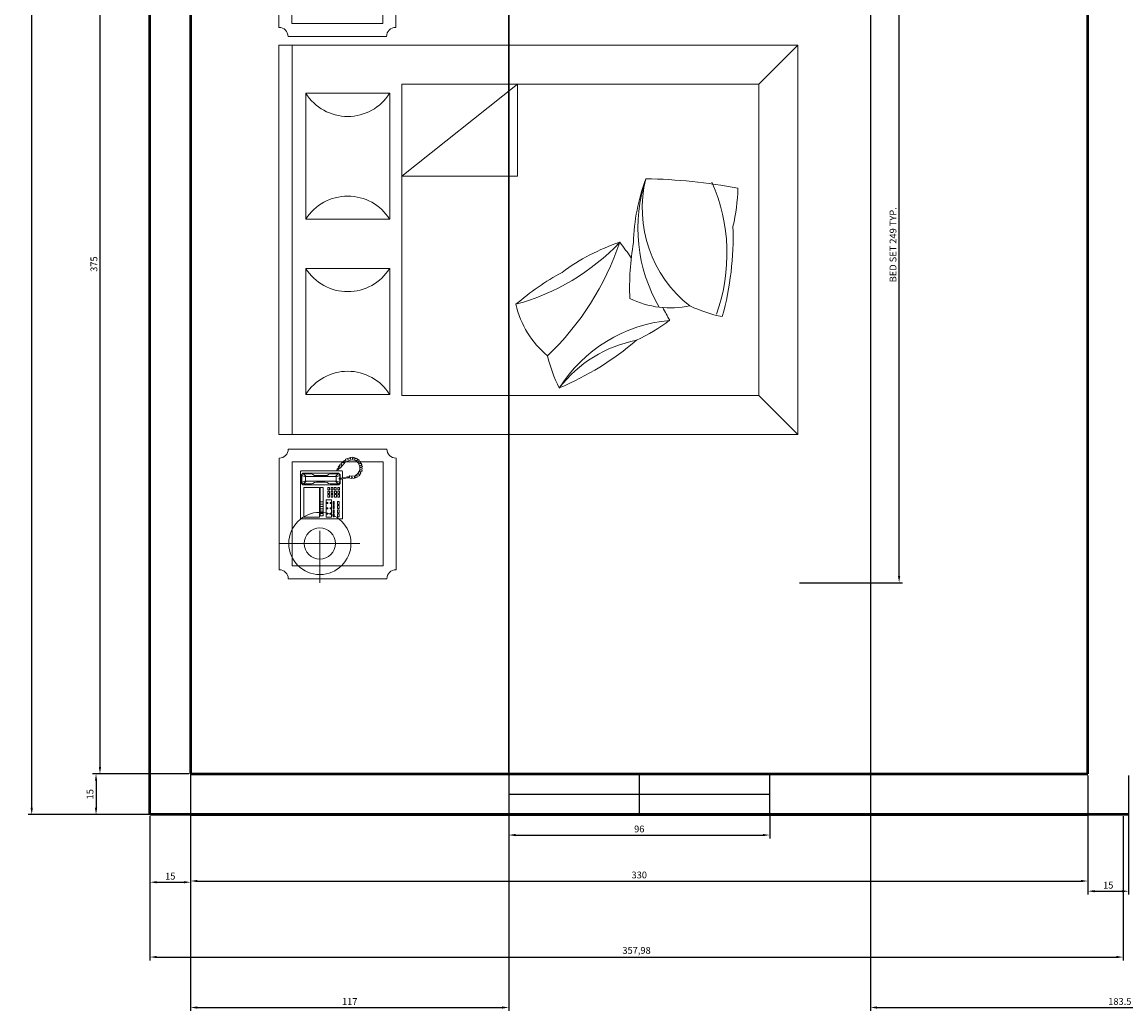
# Model space of a CAD drawing. Units: inches. Extents: x 604 to 3492, y -123 to 1737.
# Tile 5 of 20: x 1528 to 1934, y 216 to 579. Entities that reach past the tile are written whole.
import ezdxf

# ---------------------------------------------------------------- set-up
doc = ezdxf.new("R2010")
doc.units = ezdxf.units.IN
for name, color, linetype, lineweight in [('A-ANNO-DIMS', 2, 'Continuous', 18), ('A-FURN', 8, 'Continuous', 18), ('A-GLAZ', 4, 'Continuous', 25), ('A-WALL', 7, 'Continuous', 50)]:
    doc.layers.add(name, color=color, linetype=linetype, lineweight=lineweight)
doc.styles.get("Standard").update_dxf_attribs({"font": 'arial.ttf'})
doc.dimstyles.new('ISO-25', dxfattribs={"dimtxt": 2.5, "dimasz": 2.5, "dimexe": 1.25, "dimexo": 0.625, "dimtad": 1, "dimtxsty": 'Standard', "dimcen": 2.5, "dimadec": 0, "dimazin": 0, "dimtfac": 1, "dimtmove": 0, "dimatfit": 3, "dimfxl": 1, "dimarcsym": 0})

# ---------------------------------------------------------------- blocks, each defined once
blk = doc.blocks.new('A$C50B66110')
for p, q in [((0.5716, 1.9488), (0.5716, 2)), ((0.5716, 2), (2.0719, 2)), ((2.0719, 1.9488), (2.0719, 2)), ((0.0153, 1.9631), (0.0153, 1.5831)), ((0.0503, 1.9981), (0.4803, 1.9981)), ((0.1513, 1.6871), (0.1513, 1.9967)), ((0.5153, 1.9631), (0.5153, 1.5831)), ((2.1051, 1.9643), (2.1051, 1.5843)), ((2.5701, 1.9993), (2.1401, 1.9993)), ((2.6051, 1.9643), (2.6051, 1.5843)), ((0.0653, 1.9481), (0.0653, 1.5981)), ((0.0653, 1.9481), (0.4653, 1.9481)), ((0.4653, 1.9481), (0.4653, 1.5981)), ((2.0719, 1.9488), (0.5716, 1.9488)), ((0.5716, 1.9488), (0.5716, 0)), ((2.0719, 0), (2.0719, 1.9488)), ((2.1551, 1.9493), (2.1551, 1.5993)), ((2.5551, 1.9493), (2.1551, 1.9493)), ((2.3505, 1.62), (2.3505, 1.9295)), ((2.5551, 1.9493), (2.5551, 1.5993)), ((0.7257, 1.5725), (0.7257, 1.8954)), ((0.7257, 1.8954), (1.2113, 1.8954)), ((1.2113, 1.8954), (1.2113, 1.5725)), ((1.4007, 1.5725), (1.4007, 1.8954)), ((1.4007, 1.8954), (1.8863, 1.8954)), ((1.8863, 1.8954), (1.8863, 1.5725)), ((0, 1.8416), (0.2001, 1.8416)), ((2.5018, 1.7744), (2.2017, 1.7744)), ((0.0653, 1.5981), (0.4653, 1.5981)), ((2.5551, 1.5993), (2.1551, 1.5993)), ((0.0503, 1.5481), (0.4803, 1.5481)), ((1.2113, 1.5725), (0.7257, 1.5725)), ((1.8863, 1.5725), (1.4007, 1.5725)), ((2.5701, 1.5493), (2.1401, 1.5493)), ((1.5665, 1.5254), (1.5665, 1.0802)), ((1.5665, 1.5254), (1.9219, 1.0802)), ((1.9219, 1.0802), (1.5665, 1.0802)), ((0.5716, 0), (0.7216, 0.15)), ((2.0719, 0), (1.9219, 0.15)), ((0.5716, 0), (2.0719, 0))]:
    blk.add_line(p, q)
at = {"linetype": 'ByBlock'}
for p, q in [((0.2481, 1.9162), (0.2458, 1.9139)), ((0.2481, 1.9162), (0.4287, 1.9162)), ((0.4287, 1.9162), (0.4309, 1.9139)), ((0.2458, 1.9139), (0.2458, 1.7562)), ((0.2526, 1.9036), (0.2526, 1.8431)), ((0.3669, 1.9036), (0.2526, 1.9036)), ((0.3669, 1.8431), (0.3669, 1.9036)), ((0.3772, 1.9071), (0.3818, 1.9128)), ((0.3772, 1.7688), (0.3772, 1.9071)), ((0.3818, 1.9094), (0.3807, 1.9048)), ((0.3807, 1.9048), (0.3807, 1.8739)), ((0.3807, 1.9048), (0.3909, 1.8945)), ((0.3807, 1.8739), (0.3829, 1.8682)), ((0.3818, 1.9128), (0.4161, 1.9128)), ((0.3864, 1.9116), (0.3818, 1.9094)), ((0.3921, 1.8968), (0.3864, 1.9116)), ((0.3864, 1.9116), (0.4138, 1.9116)), ((0.3909, 1.8945), (0.3921, 1.8968)), ((0.3909, 1.8431), (0.3909, 1.8945)), ((0.4081, 1.8968), (0.3921, 1.8968)), ((0.4081, 1.8968), (0.4138, 1.9116)), ((0.4092, 1.8945), (0.4081, 1.8968)), ((0.4195, 1.9048), (0.4092, 1.8945)), ((0.4092, 1.8431), (0.4092, 1.8945)), ((0.4138, 1.9116), (0.4184, 1.9094)), ((0.4161, 1.9128), (0.4218, 1.9071)), ((0.4195, 1.8739), (0.4172, 1.8682)), ((0.4184, 1.9094), (0.4195, 1.9048)), ((0.4195, 1.9048), (0.4195, 1.8739)), ((0.4218, 1.9071), (0.4218, 1.7699)), ((0.4309, 1.9139), (0.4309, 1.7562)), ((0.2526, 1.8431), (0.3669, 1.8431)), ((0.2572, 1.8408), (0.2572, 1.8294)), ((0.3669, 1.8408), (0.2572, 1.8408)), ((0.2572, 1.8294), (0.3669, 1.8294)), ((0.2664, 1.8408), (0.2664, 1.8294)), ((0.2755, 1.8408), (0.2755, 1.8294)), ((0.2846, 1.8408), (0.2846, 1.8294)), ((0.2938, 1.8408), (0.2938, 1.8294)), ((0.3029, 1.8408), (0.3029, 1.8294)), ((0.3121, 1.8408), (0.3121, 1.8294)), ((0.3669, 1.8294), (0.3669, 1.8408)), ((0.3829, 1.8682), (0.3864, 1.8625)), ((0.3864, 1.8625), (0.3875, 1.8545)), ((0.3875, 1.8545), (0.3875, 1.8431)), ((0.3875, 1.8214), (0.3875, 1.8431)), ((0.3909, 1.8431), (0.3909, 1.7813)), ((0.4092, 1.8431), (0.4092, 1.7813)), ((0.4138, 1.8625), (0.4127, 1.8545)), ((0.4127, 1.8545), (0.4127, 1.8431)), ((0.4127, 1.8214), (0.4127, 1.8431)), ((0.4172, 1.8682), (0.4138, 1.8625)), ((0.3201, 1.8168), (0.2526, 1.8168)), ((0.2526, 1.8168), (0.2526, 1.7962)), ((0.2526, 1.7962), (0.3201, 1.7962)), ((0.2652, 1.7905), (0.2538, 1.7905)), ((0.2538, 1.7905), (0.2538, 1.7859)), ((0.2675, 1.8145), (0.2641, 1.8145)), ((0.2641, 1.8145), (0.2641, 1.8111)), ((0.2641, 1.8111), (0.2675, 1.8111)), ((0.2641, 1.8019), (0.2641, 1.7985)), ((0.2675, 1.8019), (0.2641, 1.8019)), ((0.2641, 1.7985), (0.2675, 1.7985)), ((0.2652, 1.7859), (0.2652, 1.7905)), ((0.2675, 1.8111), (0.2675, 1.8145)), ((0.2675, 1.7985), (0.2675, 1.8019)), ((0.2812, 1.7905), (0.2698, 1.7905)), ((0.2698, 1.7905), (0.2698, 1.7859)), ((0.2812, 1.7859), (0.2812, 1.7905)), ((0.2846, 1.8145), (0.2846, 1.8111)), ((0.2881, 1.8145), (0.2846, 1.8145)), ((0.2846, 1.8111), (0.2881, 1.8111)), ((0.2846, 1.8019), (0.2846, 1.7985)), ((0.2881, 1.8019), (0.2846, 1.8019)), ((0.2846, 1.7985), (0.2881, 1.7985)), ((0.2972, 1.7905), (0.2858, 1.7905)), ((0.2858, 1.7905), (0.2858, 1.7859)), ((0.2881, 1.8111), (0.2881, 1.8145)), ((0.2881, 1.7985), (0.2881, 1.8019)), ((0.2972, 1.7859), (0.2972, 1.7905)), ((0.3018, 1.7905), (0.3018, 1.7859)), ((0.3132, 1.7905), (0.3018, 1.7905)), ((0.3052, 1.8145), (0.3052, 1.8111)), ((0.3086, 1.8145), (0.3052, 1.8145)), ((0.3052, 1.8111), (0.3086, 1.8111)), ((0.3052, 1.8019), (0.3052, 1.7985)), ((0.3086, 1.8019), (0.3052, 1.8019)), ((0.3052, 1.7985), (0.3086, 1.7985)), ((0.3086, 1.8111), (0.3086, 1.8145)), ((0.3086, 1.7985), (0.3086, 1.8019)), ((0.3132, 1.7859), (0.3132, 1.7905)), ((0.3201, 1.7962), (0.3201, 1.8168)), ((0.3304, 1.8111), (0.3395, 1.8111)), ((0.3304, 1.8042), (0.3304, 1.8111)), ((0.3395, 1.8042), (0.3304, 1.8042)), ((0.3304, 1.7985), (0.3395, 1.7985)), ((0.3304, 1.7916), (0.3304, 1.7985)), ((0.3395, 1.7916), (0.3304, 1.7916)), ((0.3395, 1.8111), (0.3395, 1.8042)), ((0.3395, 1.7985), (0.3395, 1.7916)), ((0.3441, 1.8042), (0.3441, 1.8111)), ((0.3441, 1.8111), (0.3532, 1.8111)), ((0.3532, 1.8042), (0.3441, 1.8042)), ((0.3441, 1.7985), (0.3532, 1.7985)), ((0.3441, 1.7916), (0.3441, 1.7985)), ((0.3532, 1.7916), (0.3441, 1.7916)), ((0.3532, 1.8111), (0.3532, 1.8042)), ((0.3532, 1.7985), (0.3532, 1.7916)), ((0.3578, 1.8111), (0.3669, 1.8111)), ((0.3578, 1.8042), (0.3578, 1.8111)), ((0.3669, 1.8042), (0.3578, 1.8042)), ((0.3578, 1.7985), (0.3669, 1.7985)), ((0.3578, 1.7916), (0.3578, 1.7985)), ((0.3669, 1.7916), (0.3578, 1.7916)), ((0.3669, 1.8111), (0.3669, 1.8042)), ((0.3669, 1.7985), (0.3669, 1.7916)), ((0.3807, 1.8019), (0.3829, 1.8076)), ((0.3807, 1.7711), (0.3807, 1.8019)), ((0.3829, 1.8076), (0.3864, 1.8134)), ((0.3864, 1.8134), (0.3875, 1.8214)), ((0.4138, 1.8134), (0.4127, 1.8214)), ((0.4172, 1.8076), (0.4138, 1.8134)), ((0.4195, 1.8019), (0.4172, 1.8076)), ((0.4195, 1.7711), (0.4195, 1.8019)), ((0.2458, 1.7562), (0.2481, 1.7539)), ((0.4, 1.7539), (0.2481, 1.7539)), ((0.2538, 1.7859), (0.2652, 1.7859)), ((0.2538, 1.7665), (0.2538, 1.7733)), ((0.2538, 1.7733), (0.2652, 1.7733)), ((0.2652, 1.7665), (0.2538, 1.7665)), ((0.2652, 1.7733), (0.2652, 1.7665)), ((0.2698, 1.7859), (0.2812, 1.7859)), ((0.2698, 1.7665), (0.2698, 1.7733)), ((0.2698, 1.7733), (0.2812, 1.7733)), ((0.2812, 1.7665), (0.2698, 1.7665)), ((0.2812, 1.7733), (0.2812, 1.7665)), ((0.2858, 1.7859), (0.2972, 1.7859)), ((0.2858, 1.7665), (0.2858, 1.7733)), ((0.2858, 1.7733), (0.2972, 1.7733)), ((0.2972, 1.7665), (0.2858, 1.7665)), ((0.2972, 1.7733), (0.2972, 1.7665)), ((0.3018, 1.7859), (0.3132, 1.7859)), ((0.3018, 1.7733), (0.3132, 1.7733)), ((0.3018, 1.7665), (0.3018, 1.7733)), ((0.3132, 1.7665), (0.3018, 1.7665)), ((0.3132, 1.7733), (0.3132, 1.7665)), ((0.3304, 1.7779), (0.3304, 1.7848)), ((0.3304, 1.7848), (0.3395, 1.7848)), ((0.3395, 1.7779), (0.3304, 1.7779)), ((0.3304, 1.7722), (0.3395, 1.7722)), ((0.3304, 1.7653), (0.3304, 1.7722)), ((0.3395, 1.7653), (0.3304, 1.7653)), ((0.3395, 1.7848), (0.3395, 1.7779)), ((0.3395, 1.7722), (0.3395, 1.7653)), ((0.3441, 1.7779), (0.3441, 1.7848)), ((0.3441, 1.7848), (0.3532, 1.7848)), ((0.3532, 1.7779), (0.3441, 1.7779)), ((0.3441, 1.7722), (0.3532, 1.7722)), ((0.3441, 1.7653), (0.3441, 1.7722)), ((0.3532, 1.7653), (0.3441, 1.7653)), ((0.3532, 1.7848), (0.3532, 1.7779)), ((0.3532, 1.7722), (0.3532, 1.7653)), ((0.3578, 1.7791), (0.3578, 1.7859)), ((0.3578, 1.7859), (0.3669, 1.7859)), ((0.3669, 1.7791), (0.3578, 1.7791)), ((0.3578, 1.7653), (0.3578, 1.7722)), ((0.3578, 1.7722), (0.3669, 1.7722)), ((0.3669, 1.7653), (0.3578, 1.7653)), ((0.3669, 1.7859), (0.3669, 1.7791)), ((0.3669, 1.7722), (0.3669, 1.7653)), ((0.3829, 1.7631), (0.3772, 1.7688)), ((0.3807, 1.7711), (0.3909, 1.7813)), ((0.3818, 1.7665), (0.3807, 1.7711)), ((0.3864, 1.7642), (0.3818, 1.7665)), ((0.399, 1.7631), (0.3829, 1.7631)), ((0.3921, 1.7791), (0.3864, 1.7642)), ((0.3864, 1.7642), (0.399, 1.7642)), ((0.3909, 1.7813), (0.3921, 1.7791)), ((0.4081, 1.7791), (0.3921, 1.7791)), ((0.4024, 1.7676), (0.3989, 1.7676)), ((0.3989, 1.7676), (0.3991, 1.7578)), ((0.3991, 1.7578), (0.4019, 1.7462)), ((0.4019, 1.7462), (0.4047, 1.7353)), ((0.403, 1.7585), (0.4024, 1.7676)), ((0.4026, 1.7642), (0.4138, 1.7642)), ((0.4161, 1.7631), (0.4027, 1.7631)), ((0.4047, 1.7511), (0.403, 1.7585)), ((0.4287, 1.7539), (0.404, 1.7539)), ((0.4074, 1.7402), (0.4047, 1.7511)), ((0.4092, 1.7813), (0.4081, 1.7791)), ((0.4081, 1.7791), (0.4138, 1.7642)), ((0.4195, 1.7711), (0.4092, 1.7813)), ((0.4138, 1.7642), (0.4184, 1.7665)), ((0.4218, 1.7699), (0.4161, 1.7631)), ((0.4184, 1.7665), (0.4195, 1.7711)), ((0.4309, 1.7562), (0.4287, 1.7539)), ((0.4378, 1.7742), (0.4309, 1.7768)), ((0.4309, 1.7722), (0.436, 1.7708)), ((0.436, 1.7708), (0.4406, 1.7672)), ((0.441, 1.771), (0.4378, 1.7742)), ((0.4406, 1.7672), (0.4418, 1.7656)), ((0.4434, 1.7688), (0.441, 1.771)), ((0.4443, 1.7658), (0.4418, 1.7633)), ((0.4418, 1.7656), (0.4443, 1.7658)), ((0.4418, 1.7633), (0.4511, 1.7551)), ((0.4477, 1.7704), (0.4434, 1.7688)), ((0.4497, 1.7684), (0.4477, 1.7704)), ((0.4481, 1.765), (0.4497, 1.7684)), ((0.4509, 1.7672), (0.4481, 1.765)), ((0.4539, 1.764), (0.4509, 1.7672)), ((0.4511, 1.7551), (0.4662, 1.7422)), ((0.4515, 1.7573), (0.4539, 1.764)), ((0.4577, 1.7605), (0.4515, 1.7573)), ((0.463, 1.7555), (0.4577, 1.7605)), ((0.4618, 1.7482), (0.463, 1.7555)), ((0.467, 1.7515), (0.4618, 1.7482)), ((0.4714, 1.7468), (0.467, 1.7515)), ((0.4696, 1.7418), (0.4714, 1.7468)), ((0.4026, 1.7254), (0.4021, 1.7198)), ((0.4021, 1.7198), (0.4088, 1.7187)), ((0.4088, 1.7187), (0.4023, 1.7147)), ((0.4023, 1.7147), (0.4028, 1.7085)), ((0.4051, 1.7279), (0.4026, 1.7254)), ((0.4028, 1.7085), (0.4102, 1.7078)), ((0.4102, 1.7078), (0.4037, 1.7027)), ((0.4037, 1.7027), (0.4067, 1.6974)), ((0.4047, 1.7353), (0.4044, 1.7293)), ((0.4044, 1.7293), (0.4051, 1.7279)), ((0.4081, 1.7346), (0.4074, 1.7402)), ((0.4079, 1.7286), (0.4081, 1.7346)), ((0.4121, 1.7256), (0.4079, 1.7286)), ((0.4111, 1.7203), (0.4121, 1.7256)), ((0.4123, 1.7057), (0.4111, 1.7203)), ((0.4211, 1.6946), (0.4123, 1.7057)), ((0.4708, 1.7027), (0.4606, 1.6927)), ((0.4664, 1.7418), (0.4741, 1.72)), ((0.4766, 1.7425), (0.4697, 1.7418)), ((0.4741, 1.72), (0.4708, 1.7027)), ((0.472, 1.733), (0.4787, 1.7356)), ((0.4794, 1.7332), (0.472, 1.733)), ((0.4743, 1.7075), (0.4815, 1.7073)), ((0.4798, 1.7013), (0.4743, 1.7075)), ((0.4761, 1.7233), (0.481, 1.7279)), ((0.4824, 1.7233), (0.4761, 1.7233)), ((0.4764, 1.7154), (0.4835, 1.7175)), ((0.4824, 1.7119), (0.4764, 1.7154)), ((0.4787, 1.7356), (0.4766, 1.7425)), ((0.481, 1.7279), (0.4794, 1.7332)), ((0.4815, 1.7073), (0.4824, 1.7119)), ((0.4835, 1.7175), (0.4824, 1.7233)), ((0.4067, 1.6974), (0.4137, 1.6988)), ((0.4137, 1.6988), (0.4104, 1.6923)), ((0.4104, 1.6923), (0.4139, 1.6881)), ((0.4139, 1.6881), (0.4192, 1.692)), ((0.4192, 1.692), (0.4183, 1.6858)), ((0.4183, 1.6858), (0.4227, 1.683)), ((0.4333, 1.6881), (0.4211, 1.6946)), ((0.4227, 1.683), (0.4283, 1.6876)), ((0.4283, 1.6876), (0.4276, 1.68)), ((0.4276, 1.68), (0.4324, 1.6786)), ((0.4324, 1.6786), (0.4354, 1.6849)), ((0.4472, 1.6869), (0.4333, 1.6881)), ((0.4354, 1.6849), (0.4382, 1.6786)), ((0.4382, 1.6786), (0.4421, 1.6782)), ((0.4421, 1.6782), (0.4437, 1.6849)), ((0.4437, 1.6849), (0.4463, 1.6775)), ((0.4463, 1.6775), (0.4507, 1.6786)), ((0.4606, 1.6927), (0.4472, 1.6869)), ((0.4507, 1.6786), (0.4509, 1.6849)), ((0.4509, 1.6849), (0.4562, 1.6802)), ((0.4562, 1.6802), (0.4599, 1.6821)), ((0.4592, 1.689), (0.4641, 1.683)), ((0.4599, 1.6821), (0.4592, 1.689)), ((0.4641, 1.683), (0.4678, 1.6863)), ((0.465, 1.6925), (0.4715, 1.6897)), ((0.4678, 1.6863), (0.465, 1.6925)), ((0.4745, 1.6925), (0.4713, 1.6988)), ((0.4713, 1.6988), (0.478, 1.6967)), ((0.4715, 1.6897), (0.4745, 1.6925)), ((0.478, 1.6967), (0.4798, 1.7013)), ((0.7216, 1.5254), (1.9219, 1.5254)), ((0.7216, 1.5254), (0.7216, 0.15)), ((1.9219, 0.15), (1.9219, 1.5254)), ((0.7216, 0.15), (1.9219, 0.15))]:
    blk.add_line(p, q, dxfattribs=at)
for centre, radius in [((0.1513, 1.8416), 0.12), ((0.1513, 1.8416), 0.06), ((2.3505, 1.7744), 0.12), ((2.3505, 1.7744), 0.06)]:
    blk.add_circle(centre, radius)
for centre, radius, start, end in [((0.0153, 1.9981), 0.035, 270, 0), ((0.5153, 1.9981), 0.035, 180, 270), ((2.1051, 1.9993), 0.035, 270, 0), ((2.6051, 1.9993), 0.035, 180, 270), ((0.6244, 1.734), 0.1906, 302.1202, 57.8798), ((1.3126, 1.734), 0.1906, 122.1202, 237.8798), ((1.2994, 1.734), 0.1906, 302.1202, 57.8798), ((1.9876, 1.734), 0.1906, 122.1202, 237.8798), ((0.0153, 1.5481), 0.035, 0, 90), ((0.5153, 1.5481), 0.035, 90, 180), ((2.1051, 1.5493), 0.035, 0, 90), ((2.6051, 1.5493), 0.035, 90, 180), ((1.1502, 0.7366), 0.3575, 102.4782, 140.4625), ((0.328, 0.4368), 0.9879, 28.4971, 41.0566), ((1.9117, 1.3157), 0.8697, 195.336, 226.4193), ((0.9996, 0.4307), 0.548, 103.2034, 117.0362), ((1.656, 1.7093), 1.0798, 223.6306, 251.4288), ((0.4482, 0.4408), 0.5655, 5.3391, 57.6895), ((1.8226, 1.3753), 1.1652, 203.0642, 220.3209), ((0.4548, 0.5307), 0.4879, 10.6986, 52.6864), ((0.5648, 0.4378), 0.7874, 18.3527, 36.6851), ((-0.0179, 2.4352), 2.1977, 305.2966, 307.2418), ((1.4166, 0.4903), 0.3575, 154.0418, 192.0262), ((1.1403, -0.3401), 0.9879, 80.0607, 92.6202), ((1.5981, 0.9345), 0.734, 205.259, 216.9351), ((1.3672, 0.0075), 0.6085, 71.81, 120.1351), ((1.4431, 0.1219), 0.4774, 76.1849, 142.0017), ((1.2867, -0.154), 0.7874, 69.9163, 88.2487), ((-0.6401, 0.6314), 2.1977, 349.4884, 358.8054), ((-0.0179, 2.4352), 2.1977, 297.9248, 299.3793), ((1.5626, 0.1822), 0.548, 154.767, 168.5998), ((1.2678, 0.9611), 0.6885, 250.2936, 293.6414), ((1.3343, 1.4141), 1.1652, 254.6278, 271.8845), ((1.5399, 0.9642), 0.734, 256.8226, 268.4988)]:
    blk.add_arc(centre, radius, start, end)
blk = doc.blocks.new('*D54')
at = {"layer": 'A-ANNO-DIMS', "color": 0, "lineweight": -2, "transparency": 16777216}
for p, q in [((1919.57, 302.08), (1919.57, 258.28)), ((1934.57, 302.08), (1934.57, 258.28)), ((1922.07, 259.53), (1932.07, 259.53))]:
    blk.add_line(p, q, dxfattribs=at)
at = {"layer": 'A-ANNO-DIMS', "color": 0, "transparency": 16777216}
for points in [[(1922.07, 259.95), (1922.07, 259.11), (1919.57, 259.53)], [(1932.07, 259.95), (1932.07, 259.11), (1934.57, 259.53)]]:
    blk.add_solid(points, dxfattribs=at)
at = {"layer": 'Defpoints', "color": 0, "transparency": 16777216}
for p in [(1919.57, 302.7), (1934.57, 302.7), (1934.57, 259.53)]:
    blk.add_point(p, dxfattribs=at)
at = {"layer": 'A-ANNO-DIMS', "color": 0, "transparency": 16777216, "insert": (1927.07, 261.43), "char_height": 2.5, "attachment_point": 5}
blk.add_mtext('15', dxfattribs=at)
blk = doc.blocks.new('*D55')
at = {"layer": 'A-ANNO-DIMS', "color": 0, "lineweight": -2, "transparency": 16777216}
for p, q in [((1589.57, 302.08), (1589.57, 262.03)), ((1919.57, 302.08), (1919.57, 262.03)), ((1592.07, 263.28), (1917.07, 263.28))]:
    blk.add_line(p, q, dxfattribs=at)
at = {"layer": 'A-ANNO-DIMS', "color": 0, "transparency": 16777216}
for points in [[(1592.07, 263.7), (1592.07, 262.86), (1589.57, 263.28)], [(1917.07, 263.7), (1917.07, 262.86), (1919.57, 263.28)]]:
    blk.add_solid(points, dxfattribs=at)
at = {"layer": 'Defpoints', "color": 0, "transparency": 16777216}
for p in [(1589.57, 302.7), (1919.57, 302.7), (1919.57, 263.28)]:
    blk.add_point(p, dxfattribs=at)
at = {"layer": 'A-ANNO-DIMS', "color": 0, "transparency": 16777216, "insert": (1754.57, 265.18), "char_height": 2.5, "attachment_point": 5}
blk.add_mtext('330', dxfattribs=at)
blk = doc.blocks.new('*D56')
at = {"layer": 'A-ANNO-DIMS', "color": 0, "lineweight": -2, "transparency": 16777216}
for p, q in [((1574.57, 287.08), (1574.57, 261.59)), ((1589.57, 287.08), (1589.57, 261.59)), ((1577.07, 262.84), (1587.07, 262.84))]:
    blk.add_line(p, q, dxfattribs=at)
at = {"layer": 'A-ANNO-DIMS', "color": 0, "transparency": 16777216}
for points in [[(1577.07, 263.25), (1577.07, 262.42), (1574.57, 262.84)], [(1587.07, 263.25), (1587.07, 262.42), (1589.57, 262.84)]]:
    blk.add_solid(points, dxfattribs=at)
at = {"layer": 'Defpoints', "color": 0, "transparency": 16777216}
for p in [(1574.57, 287.7), (1589.57, 287.7), (1589.57, 262.84)]:
    blk.add_point(p, dxfattribs=at)
at = {"layer": 'A-ANNO-DIMS', "color": 0, "transparency": 16777216, "insert": (1582.07, 264.74), "char_height": 2.5, "attachment_point": 5}
blk.add_mtext('15', dxfattribs=at)
blk = doc.blocks.new('*D57')
at = {"layer": 'A-ANNO-DIMS', "color": 0, "lineweight": -2, "transparency": 16777216}
for p, q in [((1574.57, 287.08), (1574.57, 234.06)), ((1932.56, 287.08), (1932.56, 234.06)), ((1577.07, 235.31), (1930.06, 235.31))]:
    blk.add_line(p, q, dxfattribs=at)
at = {"layer": 'A-ANNO-DIMS', "color": 0, "transparency": 16777216}
for points in [[(1577.07, 235.73), (1577.07, 234.9), (1574.57, 235.31)], [(1930.06, 235.73), (1930.06, 234.9), (1932.56, 235.31)]]:
    blk.add_solid(points, dxfattribs=at)
at = {"layer": 'Defpoints', "color": 0, "transparency": 16777216}
for p in [(1574.57, 287.7), (1932.56, 287.7), (1932.56, 235.31)]:
    blk.add_point(p, dxfattribs=at)
at = {"layer": 'A-ANNO-DIMS', "color": 0, "transparency": 16777216, "insert": (1753.57, 237.44), "char_height": 2.5, "attachment_point": 5}
blk.add_mtext('357,98', dxfattribs=at)
blk = doc.blocks.new('*D58')
at = {"layer": 'A-ANNO-DIMS', "color": 0, "lineweight": -2, "transparency": 16777216}
for p, q in [((1706.57, 287.08), (1706.57, 278.94)), ((1802.57, 287.08), (1802.57, 278.94)), ((1709.07, 280.19), (1800.07, 280.19))]:
    blk.add_line(p, q, dxfattribs=at)
at = {"layer": 'A-ANNO-DIMS', "color": 0, "transparency": 16777216}
for points in [[(1709.07, 280.6), (1709.07, 279.77), (1706.57, 280.19)], [(1800.07, 280.6), (1800.07, 279.77), (1802.57, 280.19)]]:
    blk.add_solid(points, dxfattribs=at)
at = {"layer": 'Defpoints', "color": 0, "transparency": 16777216}
for p in [(1706.57, 287.7), (1802.57, 287.7), (1802.57, 280.19)]:
    blk.add_point(p, dxfattribs=at)
at = {"layer": 'A-ANNO-DIMS', "color": 0, "transparency": 16777216, "insert": (1754.57, 282.09), "char_height": 2.5, "attachment_point": 5}
blk.add_mtext('96', dxfattribs=at)
blk = doc.blocks.new('*D67')
at = {"layer": 'A-ANNO-DIMS', "color": 0, "lineweight": -2, "transparency": 16777216}
for p, q in [((1588.95, 677.7), (1554.96, 677.7)), ((1556.21, 675.2), (1556.21, 305.2)), ((1588.95, 302.7), (1554.96, 302.7))]:
    blk.add_line(p, q, dxfattribs=at)
at = {"layer": 'A-ANNO-DIMS', "color": 0, "transparency": 16777216}
for points in [[(1555.79, 675.2), (1556.62, 675.2), (1556.21, 677.7)], [(1555.79, 305.2), (1556.62, 305.2), (1556.21, 302.7)]]:
    blk.add_solid(points, dxfattribs=at)
at = {"layer": 'Defpoints', "color": 0, "transparency": 16777216}
for p in [(1589.57, 677.7), (1556.21, 302.7), (1589.57, 302.7)]:
    blk.add_point(p, dxfattribs=at)
at = {"layer": 'A-ANNO-DIMS', "color": 0, "transparency": 16777216, "insert": (1554.3, 490.2), "char_height": 2.5, "attachment_point": 5, "rotation": 90}
blk.add_mtext('375', dxfattribs=at)
blk = doc.blocks.new('*D68')
at = {"layer": 'A-ANNO-DIMS', "color": 0, "lineweight": -2, "transparency": 16777216}
for p, q in [((1588.95, 302.7), (1553.52, 302.7)), ((1554.77, 300.2), (1554.77, 290.2)), ((1588.95, 287.7), (1553.52, 287.7))]:
    blk.add_line(p, q, dxfattribs=at)
at = {"layer": 'A-ANNO-DIMS', "color": 0, "transparency": 16777216}
for points in [[(1554.36, 300.2), (1555.19, 300.2), (1554.77, 302.7)], [(1554.36, 290.2), (1555.19, 290.2), (1554.77, 287.7)]]:
    blk.add_solid(points, dxfattribs=at)
at = {"layer": 'Defpoints', "color": 0, "transparency": 16777216}
for p in [(1589.57, 302.7), (1554.77, 287.7), (1589.57, 287.7)]:
    blk.add_point(p, dxfattribs=at)
at = {"layer": 'A-ANNO-DIMS', "color": 0, "transparency": 16777216, "insert": (1552.87, 295.2), "char_height": 2.5, "attachment_point": 5, "rotation": 90}
blk.add_mtext('15', dxfattribs=at)
blk = doc.blocks.new('*D69')
at = {"layer": 'A-ANNO-DIMS', "color": 0, "lineweight": -2, "transparency": 16777216}
for p, q in [((1573.95, 1287.7), (1529.86, 1287.7)), ((1531.11, 290.2), (1531.11, 1285.2)), ((1573.95, 287.7), (1529.86, 287.7))]:
    blk.add_line(p, q, dxfattribs=at)
at = {"layer": 'A-ANNO-DIMS', "color": 0, "transparency": 16777216}
for points in [[(1530.69, 1285.2), (1531.52, 1285.2), (1531.11, 1287.7)], [(1530.69, 290.2), (1531.52, 290.2), (1531.11, 287.7)]]:
    blk.add_solid(points, dxfattribs=at)
at = {"layer": 'Defpoints', "color": 0, "transparency": 16777216}
for p in [(1531.11, 1287.7), (1574.57, 1287.7), (1574.57, 287.7)]:
    blk.add_point(p, dxfattribs=at)
at = {"layer": 'A-ANNO-DIMS', "color": 0, "transparency": 16777216, "insert": (1529.21, 787.7), "char_height": 2.5, "attachment_point": 5, "rotation": 90}
blk.add_mtext('1000', dxfattribs=at)
blk = doc.blocks.new('WIN-96')
for p, q in [((15, 96), (0, 96)), ((7.5, 96), (7.5, 0)), ((15, 96), (15, 0)), ((15, 48), (0, 48))]:
    blk.add_line(p, q)
blk.add_lwpolyline([(0, 96), (0, 0), (15, 0), (15, 96)], close=True)
blk = doc.blocks.new('*D77')
at = {"layer": 'A-ANNO-DIMS', "color": 0, "lineweight": -2, "transparency": 16777216}
for p, q in [((1813.47, 621.62), (1851.39, 621.62)), ((1850.14, 375.49), (1850.14, 619.12)), ((1813.47, 372.99), (1851.39, 372.99))]:
    blk.add_line(p, q, dxfattribs=at)
at = {"layer": 'A-ANNO-DIMS', "color": 0, "transparency": 16777216}
for points in [[(1849.72, 619.12), (1850.56, 619.12), (1850.14, 621.62)], [(1849.72, 375.49), (1850.56, 375.49), (1850.14, 372.99)]]:
    blk.add_solid(points, dxfattribs=at)
at = {"layer": 'Defpoints', "color": 0, "transparency": 16777216}
for p in [(1812.84, 621.62), (1850.14, 621.62), (1812.84, 372.99)]:
    blk.add_point(p, dxfattribs=at)
at = {"layer": 'A-ANNO-DIMS', "color": 0, "transparency": 16777216, "insert": (1848.22, 497.3), "char_height": 2.5, "attachment_point": 5, "rotation": 90}
blk.add_mtext('BED SET 249 TYP.', dxfattribs=at)
blk = doc.blocks.new('*D102')
at = {"layer": 'A-ANNO-DIMS', "color": 0, "lineweight": -2, "transparency": 16777216}
for p, q in [((1839.57, 972.08), (1839.57, 215.5)), ((2023.07, 972.08), (2023.07, 215.5)), ((1842.07, 216.75), (2020.57, 216.75))]:
    blk.add_line(p, q, dxfattribs=at)
at = {"layer": 'A-ANNO-DIMS', "color": 0, "transparency": 16777216}
for points in [[(1842.07, 217.17), (1842.07, 216.33), (1839.57, 216.75)], [(2020.57, 217.17), (2020.57, 216.33), (2023.07, 216.75)]]:
    blk.add_solid(points, dxfattribs=at)
at = {"layer": 'Defpoints', "color": 0, "transparency": 16777216}
for p in [(1839.57, 972.7), (2023.07, 972.7), (2023.07, 216.75)]:
    blk.add_point(p, dxfattribs=at)
at = {"layer": 'A-ANNO-DIMS', "color": 0, "transparency": 16777216, "insert": (1931.32, 218.65), "char_height": 2.5, "attachment_point": 5}
blk.add_mtext('183.5', dxfattribs=at)
blk = doc.blocks.new('*D103')
at = {"layer": 'A-ANNO-DIMS', "color": 0, "lineweight": -2, "transparency": 16777216}
for p, q in [((1589.57, 1272.08), (1589.57, 215.5)), ((1706.57, 1272.08), (1706.57, 215.5)), ((1592.07, 216.75), (1704.07, 216.75))]:
    blk.add_line(p, q, dxfattribs=at)
at = {"layer": 'A-ANNO-DIMS', "color": 0, "transparency": 16777216}
for points in [[(1592.07, 217.17), (1592.07, 216.33), (1589.57, 216.75)], [(1704.07, 217.17), (1704.07, 216.33), (1706.57, 216.75)]]:
    blk.add_solid(points, dxfattribs=at)
at = {"layer": 'Defpoints', "color": 0, "transparency": 16777216}
for p in [(1589.57, 1272.7), (1706.57, 1272.7), (1706.57, 216.75)]:
    blk.add_point(p, dxfattribs=at)
at = {"layer": 'A-ANNO-DIMS', "color": 0, "transparency": 16777216, "insert": (1648.07, 218.63), "char_height": 2.5, "attachment_point": 5}
blk.add_mtext('117', dxfattribs=at)
blk = doc.blocks.new('*D108')
at = {"layer": 'A-ANNO-DIMS', "color": 0, "lineweight": -2, "transparency": 16777216}
for p, q in [((1589.57, 303.33), (1589.57, 1359.9)), ((1592.07, 1358.65), (1704.07, 1358.65)), ((1706.57, 303.33), (1706.57, 1359.9))]:
    blk.add_line(p, q, dxfattribs=at)
at = {"layer": 'A-ANNO-DIMS', "color": 0, "transparency": 16777216}
for points in [[(1592.07, 1359.07), (1592.07, 1358.23), (1589.57, 1358.65)], [(1704.07, 1359.07), (1704.07, 1358.23), (1706.57, 1358.65)]]:
    blk.add_solid(points, dxfattribs=at)
at = {"layer": 'Defpoints', "color": 0, "transparency": 16777216}
for p in [(1706.57, 1358.65), (1589.57, 302.7), (1706.57, 302.7)]:
    blk.add_point(p, dxfattribs=at)
at = {"layer": 'A-ANNO-DIMS', "color": 0, "transparency": 16777216, "insert": (1648.07, 1360.53), "char_height": 2.5, "attachment_point": 5}
blk.add_mtext('117', dxfattribs=at)

msp = doc.modelspace()

# ---------------------------------------------------------------- linework, layer by layer
at = {"layer": 'A-WALL'}
for p, q in [((1574.5743, 287.7004), (1574.5743, 1287.7004)), ((1589.5743, 302.7004), (1589.5743, 677.7004)), ((1919.5743, 302.7004), (1919.5743, 677.7004)), ((1589.5743, 302.7004), (1919.5743, 302.7004)), ((1934.5743, 287.7004), (1574.5743, 287.7004)), ((1589.5743, 287.7004), (1919.5743, 287.7004))]:
    msp.add_line(p, q, dxfattribs=at)

# ---------------------------------------------------------------- block references
at = {"layer": 'A-FURN', "xscale": 95.4379570199766, "yscale": 95.4379570199766, "zscale": 95.4379570199766, "rotation": 90}
msp.add_blockref('A$C50B66110', (1812.8441, 372.993), dxfattribs=at)
at = {"layer": 'A-GLAZ', "rotation": 89.99999999999994}
msp.add_blockref('WIN-96', (1802.5743, 287.7004), dxfattribs=at)

# ---------------------------------------------------------------- dimensions: what is measured, and where the dimension line sits
at = {"layer": 'A-ANNO-DIMS'}
for base, p1, p2, override, picture, middle in [((1706.5743, 1358.6504), (1589.5743, 302.7004), (1706.5743, 302.7004), {"dimdec": 0, "dimlfac": 1, "dimrnd": 0, "dimzin": 0, "dimdsep": 46, "dimlunit": 2}, '*D108', (1648.0743, 1360.5306)), ((1706.5743, 216.7504), (1589.5743, 1272.7004), (1706.5743, 1272.7004), {"dimdec": 0, "dimlfac": 1, "dimrnd": 0, "dimzin": 0, "dimdsep": 46, "dimlunit": 2}, '*D103', (1648.0743, 218.6306)), ((2023.0743, 216.7504), (1839.5743, 972.7004), (2023.0743, 972.7004), {"dimdec": 1, "dimlfac": 1, "dimrnd": 0, "dimzin": 0, "dimdsep": 46, "dimlunit": 2}, '*D102', (1931.3243, 218.6527)), ((1919.5743, 263.2802), (1589.5743, 302.7004), (1919.5743, 302.7004), {"dimclrd": 0, "dimclre": 0, "dimclrt": 0}, '*D55', (1754.5743, 265.1825)), ((1934.5743, 259.5302), (1919.5743, 302.7004), (1934.5743, 302.7004), {"dimclrd": 0, "dimclre": 0, "dimclrt": 0}, '*D54', (1927.0743, 261.4316)), ((1589.5743, 262.8376), (1574.5743, 287.7004), (1589.5743, 287.7004), {"dimclrd": 0, "dimclre": 0, "dimclrt": 0}, '*D56', (1582.0743, 264.739)), ((1932.5576, 235.312), (1574.5743, 287.7004), (1932.5576, 287.7004), {"dimclrd": 0, "dimclre": 0, "dimclrt": 0}, '*D57', (1753.566, 237.4394)), ((1802.5743, 280.1853), (1706.5743, 287.7004), (1802.5743, 287.7004), {"dimclrd": 0, "dimclre": 0, "dimclrt": 0}, '*D58', (1754.5743, 282.0867))]:
    dim = msp.add_linear_dim(base=base, p1=p1, p2=p2, dimstyle='ISO-25', override=override, dxfattribs=at)
    dim.commit()
    dim.dimension.update_dxf_attribs({"geometry": picture, "text_midpoint": middle})
for base, p1, p2, picture, middle in [((1531.1069, 1287.7004), (1574.5743, 287.7004), (1574.5743, 1287.7004), '*D69', (1529.2055, 787.7004)), ((1556.2056, 302.7004), (1589.5743, 677.7004), (1589.5743, 302.7004), '*D67', (1554.3033, 490.2004)), ((1554.7742, 287.7004), (1589.5743, 302.7004), (1589.5743, 287.7004), '*D68', (1552.8727, 295.2004))]:
    dim = msp.add_linear_dim(base=base, p1=p1, p2=p2, angle=90, dimstyle='ISO-25', override={"dimclrd": 0, "dimclre": 0, "dimclrt": 0}, dxfattribs=at)
    dim.commit()
    dim.dimension.update_dxf_attribs({"geometry": picture, "text_midpoint": middle})
dim = msp.add_linear_dim(base=(1850.1391, 621.6186), p1=(1812.8446, 372.9886), p2=(1812.8446, 621.6186), angle=90, text='BED SET <> TYP.', dimstyle='ISO-25', override={"dimdec": 0, "dimlfac": 1, "dimrnd": 0, "dimzin": 0, "dimdsep": 46, "dimlunit": 2}, dxfattribs=at)
dim.commit()
dim.dimension.update_dxf_attribs({"geometry": '*D77', "text_midpoint": (1848.2215, 497.3036)})

doc.saveas('drawing.dxf')
